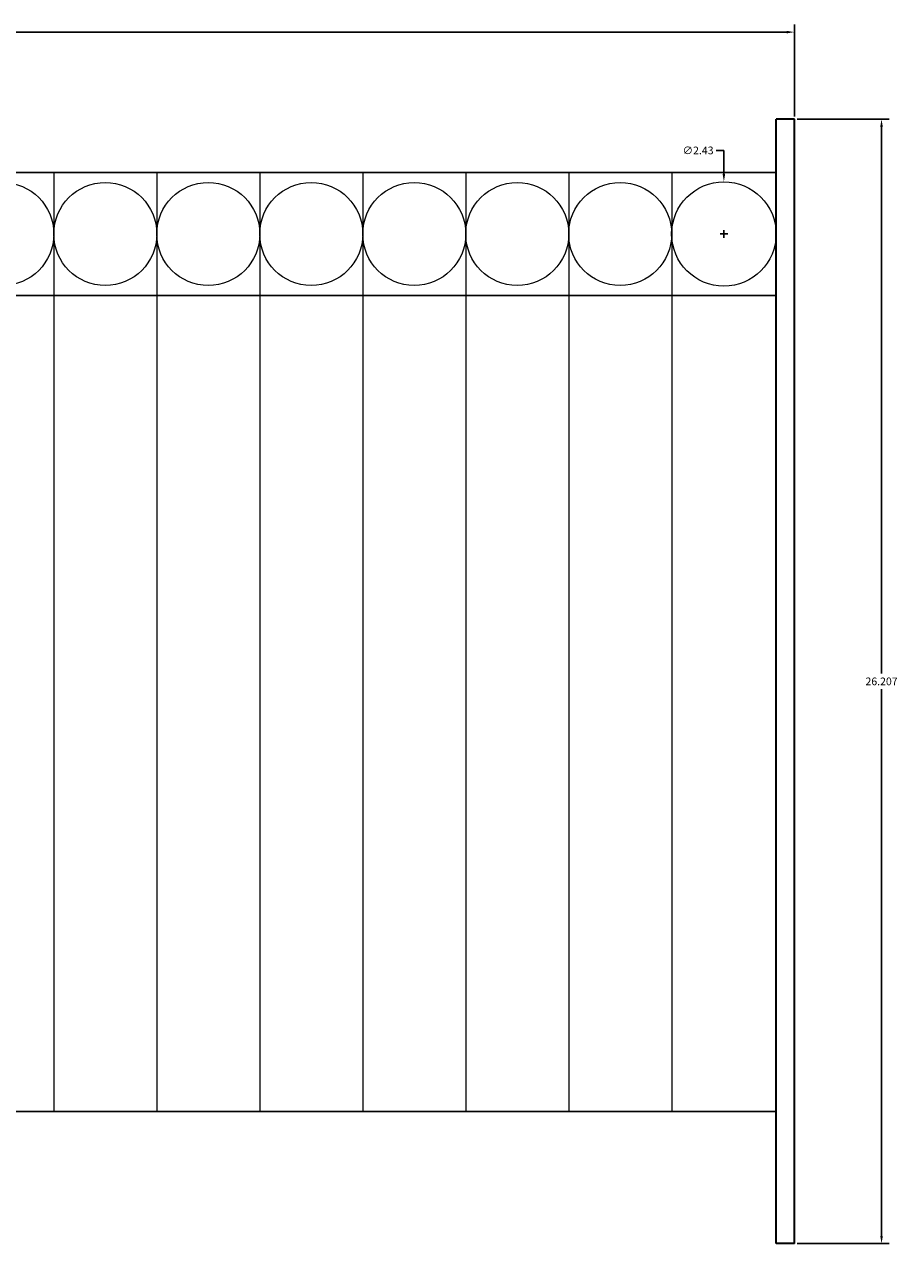
# Model space of a CAD drawing. Units: inches. Extents: x 756 to 915, y 488 to 695.
# Tile 9 of 25: x 888 to 908, y 513 to 541. Entities that reach past the tile are written whole.
import ezdxf

# ---------------------------------------------------------------- set-up
doc = ezdxf.new("R2010")
doc.units = ezdxf.units.IN
doc.header["$MEASUREMENT"] = 0
for name, color, linetype, lineweight in [('L-FENC-PCKT', 7, 'Continuous', 18), ('L-FENC-POST', 7, 'Continuous', 35), ('L-FENC-RAIL', 7, 'Continuous', 25), ('L-FENC-RING', 7, 'Continuous', 18), ('M-DIMS', 2, 'Continuous', 18)]:
    doc.layers.add(name, color=color, linetype=linetype, lineweight=lineweight)
doc.styles.get("Standard").update_dxf_attribs({"font": 'arial.ttf'})
doc.dimstyles.get("Standard").update_dxf_attribs({"dimtxt": 0.18, "dimasz": 0.18, "dimexe": 0.18, "dimexo": 0.0625, "dimgap": 0.09, "dimtad": 0, "dimtih": 1, "dimtoh": 1, "dimdec": 0, "dimzin": 0, "dimdsep": 46, "dimlunit": 3, "dimtxsty": 'Standard', "dimcen": 0.09, "dimadec": 0, "dimazin": 0, "dimtfac": 1, "dimtdec": 0, "dimtofl": 0, "dimtmove": 0, "dimatfit": 3, "dimfxl": 1, "dimtolj": 1, "dimtzin": 0, "dimarcsym": 0})

# ---------------------------------------------------------------- blocks, each defined once
blk = doc.blocks.new('FENCE-POST-RIGHT')
for p, q in [((0, 26.207), (0, 0)), ((0, 26.207), (0.427, 26.207)), ((0.427, 26.207), (0.427, 0)), ((0, 0), (0.427, 0))]:
    blk.add_line(p, q)
blk = doc.blocks.new('FENCE-PLUS-RING-BAND')
for centre, radius in [((1.286, 1.286), 1.286), ((3.773, 1.286), 1.2), ((6.173, 1.286), 1.2), ((8.572, 1.286), 1.2), ((10.972, 1.286), 1.2), ((13.372, 1.286), 1.2), ((15.772, 1.286), 1.2), ((18.172, 1.286), 1.2), ((20.572, 1.286), 1.2), ((22.972, 1.286), 1.2), ((25.372, 1.286), 1.2), ((27.772, 1.286), 1.2), ((30.172, 1.286), 1.2), ((32.572, 1.286), 1.2), ((34.971, 1.286), 1.2), ((37.388, 1.286), 1.217)]:
    blk.add_circle(centre, radius)
blk = doc.blocks.new('*D63')
at = {"layer": 'Defpoints', "color": 0, "transparency": 16777216}
for p in [(905.684, 541.143), (866.226, 539.113), (905.684, 539.113)]:
    blk.add_point(p, dxfattribs=at)
at = {"layer": 'M-DIMS', "color": 0, "lineweight": -2, "transparency": 16777216}
for p, q in [((866.226, 539.175), (866.226, 541.323)), ((866.406, 541.143), (885.561, 541.143)), ((905.504, 541.143), (886.348, 541.143)), ((905.684, 539.175), (905.684, 541.323))]:
    blk.add_line(p, q, dxfattribs=at)
at = {"layer": 'M-DIMS', "color": 0, "transparency": 16777216}
for points in [[(866.406, 541.173), (866.406, 541.113), (866.226, 541.143)], [(905.504, 541.173), (905.504, 541.113), (905.684, 541.143)]]:
    blk.add_solid(points, dxfattribs=at)
at = {"layer": 'M-DIMS', "color": 0, "transparency": 16777216, "insert": (885.955, 541.143), "char_height": 0.18, "attachment_point": 5}
blk.add_mtext('\\A1;39.46', dxfattribs=at)
blk = doc.blocks.new('*D64')
at = {"layer": 'Defpoints', "color": 0, "transparency": 16777216}
for p in [(905.684, 539.113), (907.714, 539.113), (905.684, 512.906)]:
    blk.add_point(p, dxfattribs=at)
at = {"layer": 'M-DIMS', "color": 0, "lineweight": -2, "transparency": 16777216}
for p, q in [((905.746, 539.113), (907.894, 539.113)), ((907.714, 538.933), (907.714, 526.191)), ((907.714, 513.086), (907.714, 525.828)), ((905.746, 512.906), (907.894, 512.906))]:
    blk.add_line(p, q, dxfattribs=at)
at = {"layer": 'M-DIMS', "color": 0, "transparency": 16777216}
for points in [[(907.684, 538.933), (907.744, 538.933), (907.714, 539.113)], [(907.684, 513.086), (907.744, 513.086), (907.714, 512.906)]]:
    blk.add_solid(points, dxfattribs=at)
at = {"layer": 'M-DIMS', "color": 0, "transparency": 16777216, "insert": (907.714, 526.01), "char_height": 0.18, "attachment_point": 5}
blk.add_mtext('\\A1;26.207', dxfattribs=at)
blk = doc.blocks.new('*D83')
at = {"layer": 'Defpoints', "color": 0, "transparency": 16777216}
for p in [(904.04, 537.655), (904.04, 535.221)]:
    blk.add_point(p, dxfattribs=at)
at = {"layer": 'M-DIMS', "color": 0, "lineweight": -2, "transparency": 16777216}
for p, q in [((903.86, 538.385), (904.04, 538.385)), ((904.04, 538.385), (904.04, 537.835)), ((904.04, 536.348), (904.04, 536.528)), ((903.95, 536.438), (904.13, 536.438))]:
    blk.add_line(p, q, dxfattribs=at)
at = {"layer": 'M-DIMS', "color": 0, "transparency": 16777216}
blk.add_solid([(904.07, 537.835), (904.01, 537.835), (904.04, 537.655)], dxfattribs=at)
at = {"layer": 'M-DIMS', "color": 0, "transparency": 16777216, "insert": (903.438, 538.385), "char_height": 0.18, "attachment_point": 5}
blk.add_mtext('\\A1;∅2.43', dxfattribs=at)

msp = doc.modelspace()

# ---------------------------------------------------------------- linework, layer by layer
at = {"layer": 'L-FENC-PCKT'}
for p, q in [((888.4239, 537.87), (888.4239, 515.9878)), ((890.8239, 537.87), (890.8239, 515.9878)), ((893.2238, 537.87), (893.2238, 515.9878)), ((895.6237, 537.87), (895.6237, 515.9878)), ((898.0236, 537.87), (898.0236, 515.9878)), ((900.4235, 537.87), (900.4235, 515.9878)), ((902.8234, 537.87), (902.8234, 515.9878))]:
    msp.add_line(p, q, dxfattribs=at)
at = {"layer": 'L-FENC-RAIL'}
for p, q in [((866.6522, 537.87), (905.257, 537.87)), ((866.6522, 535.0056), (905.257, 535.0056)), ((866.6522, 515.9878), (905.257, 515.9878))]:
    msp.add_line(p, q, dxfattribs=at)

# ---------------------------------------------------------------- block references
at = {"layer": 'L-FENC-POST', "rotation": 180}
msp.add_blockref('FENCE-POST-RIGHT', (905.6838, 539.113), dxfattribs=at)
at = {"layer": 'L-FENC-RING'}
msp.add_blockref('FENCE-PLUS-RING-BAND', (866.652, 535.1518), dxfattribs=at)

# ---------------------------------------------------------------- dimensions: what is measured, and where the dimension line sits
at = {"layer": 'M-DIMS'}
dim = msp.add_linear_dim(base=(905.6837, 541.1429), p1=(866.2255, 539.1129), p2=(905.6837, 539.1129), dimstyle='Standard', override={"dimdec": 2, "dimlfac": 1, "dimrnd": 0, "dimzin": 0, "dimdsep": 46, "dimlunit": 2}, dxfattribs=at)
dim.commit()
dim.dimension.update_dxf_attribs({"geometry": '*D63', "text_midpoint": (885.9546, 541.1429)})
dim = msp.add_linear_dim(base=(907.7137, 539.1129), p1=(905.6837, 512.9061), p2=(905.6837, 539.1129), angle=90, dimstyle='Standard', override={"dimdec": 3, "dimlfac": 1, "dimrnd": 0, "dimzin": 0, "dimdsep": 46, "dimlunit": 2}, dxfattribs=at)
dim.commit()
dim.dimension.update_dxf_attribs({"geometry": '*D64', "text_midpoint": (907.7137, 526.0095)})
dim = msp.add_diameter_dim_2p(p1=(904.0404, 535.221), p2=(904.04, 537.6546), dimstyle='Standard', override={"dimdec": 2, "dimlfac": 1, "dimrnd": 0, "dimzin": 0, "dimdsep": 46, "dimlunit": 2}, dxfattribs=at)
dim.commit()
dim.dimension.update_dxf_attribs({"geometry": '*D83', "text_midpoint": (903.4382, 538.3847), "dimtype": 163})

doc.saveas('drawing.dxf')
